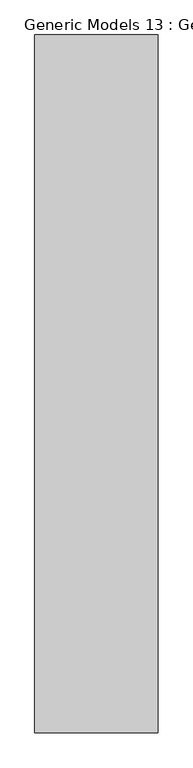
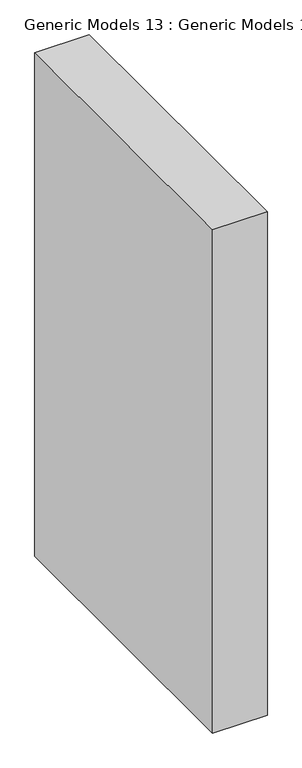
"""IFC4 building model written with IfcOpenShell, lengths in millimetres: proxy geometry, Generic Models 13 : Generic Models 13."""

from ifc_helpers import new_model, si_unit, frame, origin, place, context, project, spatial, polyline, outline, extrude, source, transform, mapped, element, save


def generic_models_13_generic_models_13_f044a1e7(model_context):
    return source(origin(), model_context, "Body", "SweptSolid", [
        extrude(outline(polyline([(913.6890071, -13286.0073314), (913.6890071, -11254.0073314), (1273.3423568, -11254.0073314), (1273.3423568, -13286.0073314), (913.6890071, -13286.0073314)])), frame((0.0, 0.0, 3200.4), z_axis=(0.0, 0.0, 1.0), x_axis=(1.0, 0.0, 0.0)), (0.0, 0.0, 1.0), 3505.2),
    ])


if __name__ == "__main__":
    model = new_model("IFC4")
    model_context = context("Model", 3, world=origin())
    ifc_project = project(units=[si_unit("LENGTHUNIT", "METRE", prefix="MILLI")], contexts=[model_context])
    site = spatial("IfcSite", under=ifc_project)
    building = spatial("IfcBuilding", under=site)
    placement = place(None, origin())
    generic_models_13_generic_models_13_shape = generic_models_13_generic_models_13_f044a1e7(model_context)
    element("IfcBuildingElementProxy", 1, Name="Generic Models 13 : Generic Models 13", ObjectType="Generic Models 13 : Generic Models 13", at=placement, inside=building, context=model_context, shape_type="MappedRepresentation", body=[
        mapped(generic_models_13_generic_models_13_shape, transform((0.0, 0.0, 0.0), x_axis=(1.0, 0.0, 0.0), y_axis=(0.0, 1.0, 0.0), z_axis=(0.0, 0.0, 1.0))),
    ])
    save(model, "model.ifc")

# Revit data of these elements
# Element 1 (IfcBuildingElementProxy, "Generic Models 13 : Generic Models 13")
#   Materials on its faces: "Clad - White"
# Materials
#   "Clad - White": class "Wood", colour RGB 242 242 238, transparency 0, Cost = 0
